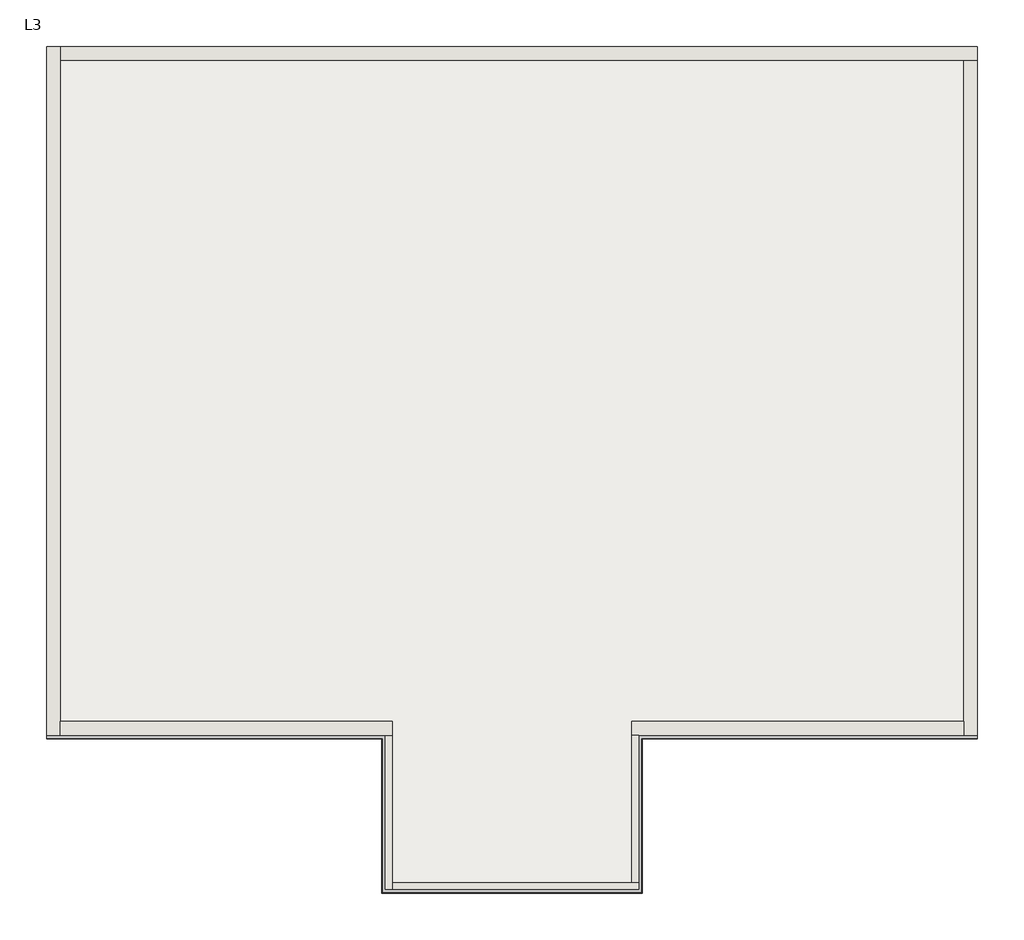
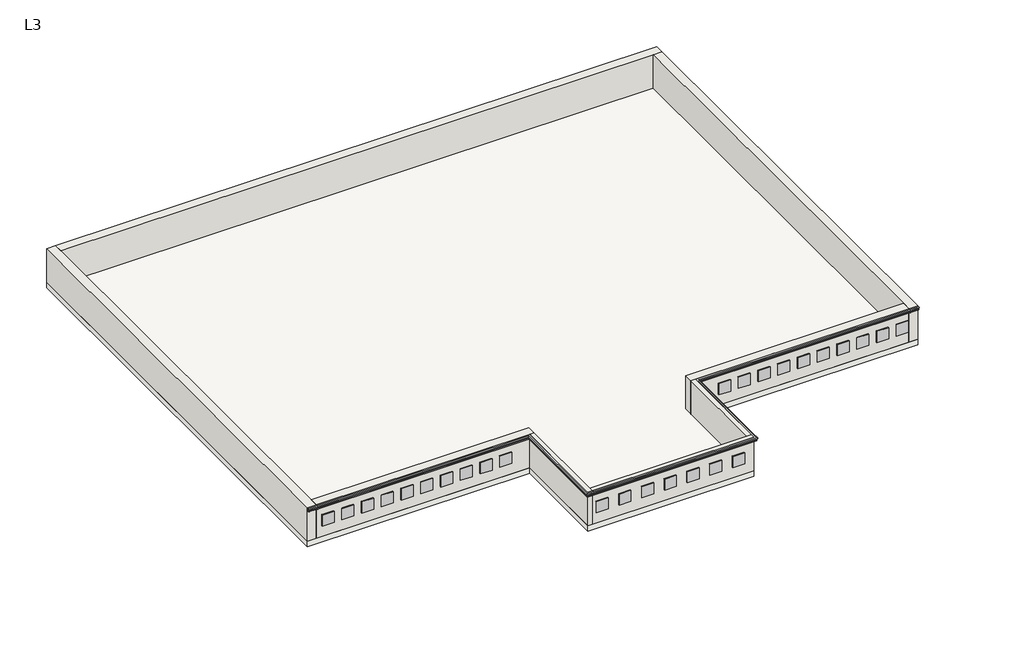
# One storey: 8 walls, 2 proxies, 1 slab.
"""IFC4 building model written with IfcOpenShell, lengths in millimetres."""

from ifc_helpers import new_model, si_unit, frame, origin, place, context, project, spatial, polyline, outline, extrude, faceted_brep, transform, mapped, element, save
from components import generic_models_17_generic_models_17_0ec560be, generic_models_18_generic_models_18_2a58dc35

model = new_model("IFC4")

# Units and contexts
model_context = context("Model", 3, world=origin())
ifc_project = project(units=[si_unit("LENGTHUNIT", "METRE", prefix="MILLI")], contexts=[model_context])

# Site, building, storey
site = spatial("IfcSite", under=ifc_project)
building = spatial("IfcBuilding", under=site)
storey = spatial("IfcBuildingStorey", under=building, Name="L3", Elevation=6527.8)

# Proxies
placement = place(None, origin())
generic_models_17_generic_models_17_shape = generic_models_17_generic_models_17_0ec560be(model_context)
element("IfcBuildingElementProxy", 1, Name="Generic Models 17 : Generic Models 17", ObjectType="Generic Models 17 : Generic Models 17", at=placement, inside=storey, context=model_context, shape_type="MappedRepresentation", body=[
    mapped(generic_models_17_generic_models_17_shape, transform((0.0, 0.0, 0.0), x_axis=(1.0, 0.0, 0.0), y_axis=(0.0, 1.0, 0.0), z_axis=(0.0, 0.0, 1.0))),
])
generic_models_18_generic_models_18_shape = generic_models_18_generic_models_18_2a58dc35(model_context)
element("IfcBuildingElementProxy", 2, Name="Generic Models 18 : Generic Models 18", ObjectType="Generic Models 18 : Generic Models 18", at=placement, inside=storey, context=model_context, shape_type="MappedRepresentation", body=[
    mapped(generic_models_18_generic_models_18_shape, transform((0.0, 0.0, 0.0), x_axis=(1.0, 0.0, 0.0), y_axis=(0.0, 1.0, 0.0), z_axis=(0.0, 0.0, 1.0))),
])

# Slab
element("IfcSlab", 3, ObjectType="6\"", at=placement, inside=storey, context=model_context, shape_type="SweptSolid", body=[
    extrude(outline(polyline([(6935.9174924, 6238.7391705), (6935.9174924, -5379.3542653), (1220.9174924, -5379.3542653), (1220.9174924, -7983.4292912), (-3046.2825076, -7983.4292912), (-3046.2825076, -5379.3542653), (-8761.2825076, -5379.3542653), (-8761.2825076, 6238.7391705), (6935.9174924, 6238.7391705)])), frame((0.0, 0.0, 6375.4), z_axis=(0.0, 0.0, 1.0), x_axis=(1.0, 0.0, 0.0)), (0.0, 0.0, 1.0), 152.4),
])

# Walls
element("IfcWall", 4, ObjectType="wall 4.5\"", at=placement, inside=storey, context=model_context, shape_type="Brep", body=[
    faceted_brep([(-3046.2825076, -5379.3542653, 6527.8), (-3046.2825076, -7983.4292912, 6527.8), (-3046.2825076, -7983.4292912, 7442.2), (-3046.2825076, -5379.3542653, 7442.2), (-2931.9825076, -5379.3542653, 6527.8), (-2931.9825076, -5379.3542653, 7442.2), (-2931.9825076, -7869.1292912, 7442.2), (-2931.9825076, -7983.4292912, 7442.2), (-2931.9825076, -7983.4292912, 6527.8), (-2931.9825076, -7869.1292912, 6527.8)], [[[0, 1, 2, 3]], [[4, 5, 6, 7, 8, 9]], [[1, 0, 4, 9, 8]], [[3, 2, 7, 6, 5]], [[0, 3, 5, 4]], [[2, 1, 8, 7]]]),
])
element("IfcWall", 5, ObjectType="wall 4.5\"", at=placement, inside=storey, context=model_context, shape_type="Brep", body=[
    faceted_brep([(-2931.9825076, -7983.4292912, 6527.8), (1220.9174924, -7983.4292912, 6527.8), (1220.9174924, -7983.4292912, 7442.2), (-2931.9825076, -7983.4292912, 7442.2), (-2931.9825076, -7869.1292912, 6527.8), (-2931.9825076, -7869.1292912, 7442.2), (1106.6174924, -7869.1292912, 7442.2), (1220.9174924, -7869.1292912, 7442.2), (1220.9174924, -7869.1292912, 6527.8), (1106.6174924, -7869.1292912, 6527.8)], [[[0, 1, 2, 3]], [[4, 5, 6, 7, 8, 9]], [[1, 0, 4, 9, 8]], [[3, 2, 7, 6, 5]], [[0, 3, 5, 4]], [[2, 1, 8, 7]]]),
])
element("IfcWall", 6, ObjectType="wall 4.5\"", at=placement, inside=storey, context=model_context, shape_type="SweptSolid", body=[
    extrude(outline(polyline([(1220.9174924, -5379.3542653), (1220.9174924, -7869.1292912), (1106.6174924, -7869.1292912), (1106.6174924, -5379.3542653), (1220.9174924, -5379.3542653)])), frame((0.0, 0.0, 6527.8), z_axis=(0.0, 0.0, 1.0), x_axis=(1.0, 0.0, 0.0)), (0.0, 0.0, 1.0), 914.4),
])
element("IfcWall", 7, ObjectType="wall 9\"", at=placement, inside=storey, context=model_context, shape_type="Brep", body=[
    faceted_brep([(-8761.2825076, 6238.7391705, 6527.8), (-8761.2825076, -5379.3542653, 6527.8), (-8761.2825076, -5379.3542653, 7442.2), (-8761.2825076, 6238.7391705, 7442.2), (-8532.6825076, 6238.7391705, 6527.8), (-8532.6825076, 6238.7391705, 7442.2), (-8532.6825076, 6010.1391705, 7442.2), (-8532.6825076, -5150.7542653, 7442.2), (-8532.6825076, -5379.3542653, 7442.2), (-8532.6825076, -5379.3542653, 6527.8), (-8532.6825076, -5150.7542653, 6527.8), (-8532.6825076, 6010.1391705, 6527.8)], [[[0, 1, 2, 3]], [[4, 5, 6, 7, 8, 9, 10, 11]], [[1, 0, 4, 11, 10, 9]], [[3, 2, 8, 7, 6, 5]], [[2, 1, 9, 8]], [[0, 3, 5, 4]]]),
])
element("IfcWall", 8, ObjectType="wall 9\"", at=placement, inside=storey, context=model_context, shape_type="Brep", body=[
    faceted_brep([(-8532.6825076, -5379.3542653, 6527.8), (-3046.2825076, -5379.3542653, 6527.8), (-2931.9825076, -5379.3542653, 6527.8), (-2931.9825076, -5379.3542653, 7442.2), (-3046.2825076, -5379.3542653, 7442.2), (-8532.6825076, -5379.3542653, 7442.2), (-8532.6825076, -5150.7542653, 6527.8), (-8532.6825076, -5150.7542653, 7442.2), (-2931.9825076, -5150.7542653, 7442.2), (-2931.9825076, -5150.7542653, 6527.8)], [[[0, 1, 2, 3, 4, 5]], [[6, 7, 8, 9]], [[2, 1, 0, 6, 9]], [[5, 4, 3, 8, 7]], [[0, 5, 7, 6]], [[3, 2, 9, 8]]]),
])
element("IfcWall", 9, ObjectType="wall 9\"", at=placement, inside=storey, context=model_context, shape_type="Brep", body=[
    faceted_brep([(-8532.6825076, 6010.1391705, 6527.8), (6707.3174924, 6010.1391705, 6527.8), (6935.9174924, 6010.1391705, 6527.8), (6935.9174924, 6010.1391705, 7442.2), (6707.3174924, 6010.1391705, 7442.2), (-8532.6825076, 6010.1391705, 7442.2), (-8532.6825076, 6238.7391705, 6527.8), (-8532.6825076, 6238.7391705, 7442.2), (6935.9174924, 6238.7391705, 7442.2), (6935.9174924, 6238.7391705, 6527.8)], [[[0, 1, 2, 3, 4, 5]], [[6, 7, 8, 9]], [[2, 1, 0, 6, 9]], [[5, 4, 3, 8, 7]], [[0, 5, 7, 6]], [[3, 2, 9, 8]]]),
])
element("IfcWall", 10, ObjectType="wall 9\"", at=placement, inside=storey, context=model_context, shape_type="Brep", body=[
    faceted_brep([(6707.3174924, 6010.1391705, 6527.8), (6707.3174924, -5150.7542653, 6527.8), (6707.3174924, -5379.3542653, 6527.8), (6707.3174924, -5379.3542653, 7442.2), (6707.3174924, -5150.7542653, 7442.2), (6707.3174924, 6010.1391705, 7442.2), (6935.9174924, 6010.1391705, 6527.8), (6935.9174924, 6010.1391705, 7442.2), (6935.9174924, -5379.3542653, 7442.2), (6935.9174924, -5379.3542653, 6527.8)], [[[0, 1, 2, 3, 4, 5]], [[6, 7, 8, 9]], [[2, 1, 0, 6, 9]], [[5, 4, 3, 8, 7]], [[0, 5, 7, 6]], [[3, 2, 9, 8]]]),
])
element("IfcWall", 11, ObjectType="wall 9\"", at=placement, inside=storey, context=model_context, shape_type="Brep", body=[
    faceted_brep([(6707.3174924, -5150.7542653, 6527.8), (1106.6174924, -5150.7542653, 6527.8), (1106.6174924, -5150.7542653, 7442.2), (6707.3174924, -5150.7542653, 7442.2), (6707.3174924, -5379.3542653, 6527.8), (6707.3174924, -5379.3542653, 7442.2), (1220.9174924, -5379.3542653, 7442.2), (1106.6174924, -5379.3542653, 7442.2), (1106.6174924, -5379.3542653, 6527.8), (1220.9174924, -5379.3542653, 6527.8)], [[[0, 1, 2, 3]], [[4, 5, 6, 7, 8, 9]], [[1, 0, 4, 9, 8]], [[3, 2, 7, 6, 5]], [[0, 3, 5, 4]], [[2, 1, 8, 7]]]),
])

save(model, "model.ifc")

# Revit data of these elements
# Type "6\""
#   Description = "Generic Floor (Material By Category), 12\" thick"
#   Assembly Code = "B1010"
#   Type Mark = "G01"
#   Function = 0
#   Layers, outside or top first: 0' - 6" no material (function 1)
# Type "wall 4.5\""
#   Description = "Generic Wall (Material By Category), 8\" thick"
#   Assembly Code = "B2010"
#   Type Mark = "G06"
#   Layers, outside or top first: 0' - 4 1/2" no material (function 1)
# Type "wall 9\""
#   Description = "Generic Wall (Material By Category), 8\" thick"
#   Assembly Code = "B2010"
#   Type Mark = "G06"
#   Layers, outside or top first: 0' - 9" no material (function 1)
# Element 1 (IfcBuildingElementProxy, "Generic Models 17 : Generic Models 17")
#   Phase Created = New Construction
# Element 2 (IfcBuildingElementProxy, "Generic Models 18 : Generic Models 18")
#   Phase Created = New Construction
# Element 3 (IfcSlab, "6\"")
#   Height Offset From Level = 0' - 0"
#   Phase Created = New Construction
#   Materials on its faces: "Default Floor"
# Elements 4, 5, 6 (IfcWall, "wall 4.5\"")
#   Top Offset = 0' - 0"
#   Base Offset = 0' - 0"
#   Unconnected Height = 3' - 0"
#   wall height = 3' - 0"
#   Phase Created = New Construction
#   Base Constraint = L3
#   Materials on its faces: "Default Wall"
# Elements 7, 8, 9, 10, 11 (IfcWall, "wall 9\"")
#   Top Offset = 0' - 0"
#   Base Offset = 0' - 0"
#   Unconnected Height = 3' - 0"
#   wall height = 3' - 0"
#   Phase Created = New Construction
#   Base Constraint = L3
#   Materials on its faces: "Default Wall"
# Materials
#   "Default Floor": colour RGB 128 128 128, transparency 0, Cost = 0
#   "Default Wall": colour RGB 192 192 192, transparency 0, Cost = 0
